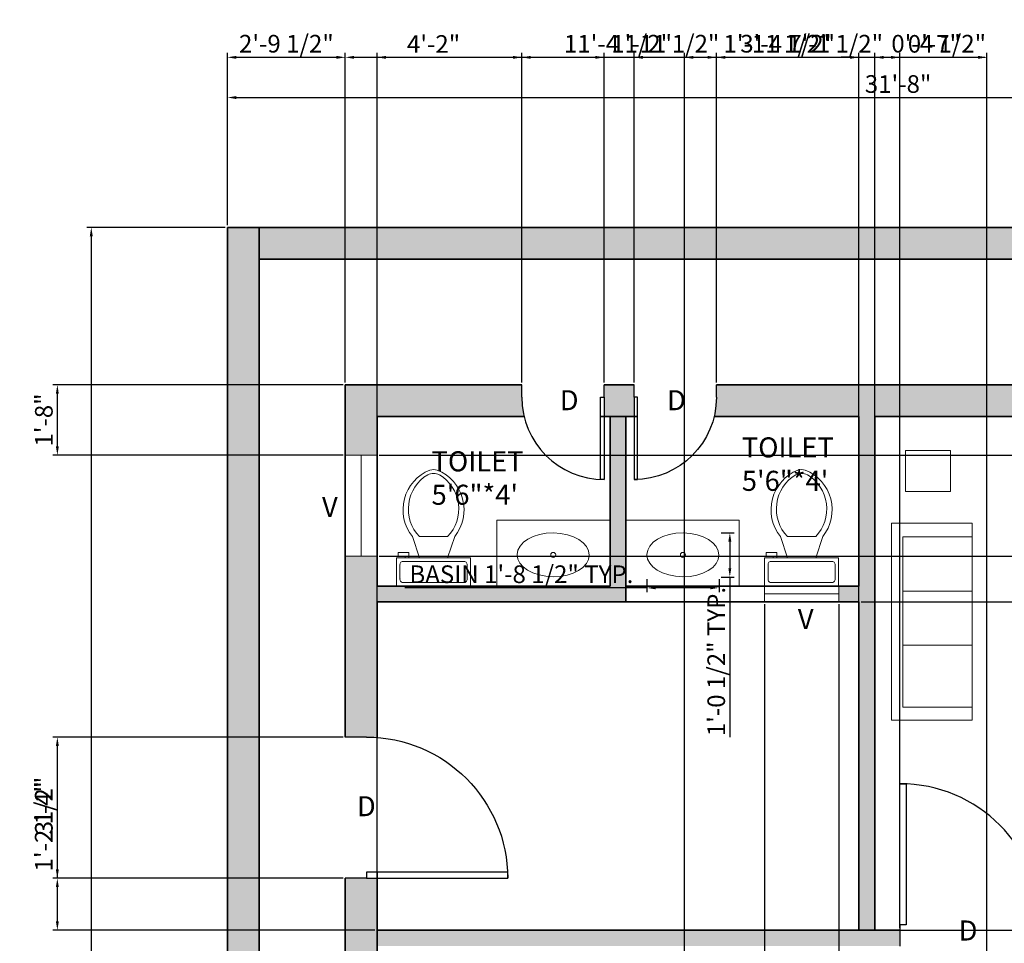
# Model space of a CAD drawing. Units: inches. Extents: x 2130 to 2621, y 981 to 1994.
# Tile 3 of 4: x 2130 to 2409, y 1732 to 1994. Entities that reach past the tile are written whole.
import ezdxf

# ---------------------------------------------------------------- set-up
doc = ezdxf.new("R2010")
doc.units = ezdxf.units.IN
for name, color, linetype, lineweight in [('A-ANNO-DIMS', 2, 'Continuous', 18), ('A-ANNO-TEXT', 10, 'Continuous', 18), ('A-AREA-IDEN', 10, 'Continuous', 18), ('A-FLOR-FIXT', 190, 'Continuous', 18), ('A-WALL-PATT', 140, 'Continuous', 13), ('C-PROP', 7, 'Continuous', 35), ('C-PROP-PATT', 140, 'Continuous', 13), ('DOOR', 130, 'Continuous', 25), ('FUR', 190, 'Continuous', 18), ('WALL', 140, 'Continuous', 35), ('WIND', 210, 'Continuous', 18)]:
    doc.layers.add(name, color=color, linetype=linetype, lineweight=lineweight)
doc.styles.get("Standard").update_dxf_attribs({"font": 'arial.ttf'})
doc.dimstyles.new('ISO-25', dxfattribs={"dimtxt": 5, "dimasz": 2.5, "dimexe": 1.25, "dimexo": 0.625, "dimtad": 1, "dimdec": 0, "dimlunit": 4, "dimtxsty": 'Standard', "dimcen": 2.5, "dimadec": 0, "dimazin": 0, "dimtfac": 1, "dimtdec": 0, "dimtmove": 0, "dimatfit": 3, "dimfxl": 1, "dimarcsym": 0})

# ---------------------------------------------------------------- blocks, each defined once
blk = doc.blocks.new('*U2')
for p, q in [((0, 0), (0, -6)), ((40, 0), (40, -6))]:
    blk.add_line(p, q)
blk.add_lwpolyline([(0, 0), (0, 40), (1.75, 40), (1.75, 0)], close=True)
blk.add_arc((0, 0), 40, 0, 90)
blk = doc.blocks.new('*D9')
at = {"layer": 'A-ANNO-DIMS', "color": 0, "lineweight": -2, "transparency": 16777216}
for p, q in [((2188.76, 1935.64), (2188.76, 1973.06)), ((2568.76, 1935.64), (2568.76, 1973.06)), ((2191.26, 1971.81), (2566.26, 1971.81))]:
    blk.add_line(p, q, dxfattribs=at)
at = {"layer": 'A-ANNO-DIMS', "color": 0, "transparency": 16777216}
for points in [[(2191.26, 1972.23), (2191.26, 1971.39), (2188.76, 1971.81)], [(2566.26, 1972.23), (2566.26, 1971.39), (2568.76, 1971.81)]]:
    blk.add_solid(points, dxfattribs=at)
at = {"layer": 'Defpoints', "color": 0, "transparency": 16777216}
for p in [(2568.76, 1971.81), (2188.76, 1935.02), (2568.76, 1935.02)]:
    blk.add_point(p, dxfattribs=at)
at = {"layer": 'A-ANNO-DIMS', "color": 0, "transparency": 16777216, "insert": (2378.76, 1974.99), "char_height": 5, "attachment_point": 5}
blk.add_mtext('31\'-8"', dxfattribs=at)
blk = doc.blocks.new('*D10')
at = {"layer": 'A-ANNO-DIMS', "color": 0, "lineweight": -2, "transparency": 16777216}
for p, q in [((2188.13, 1935.02), (2148.94, 1935.02)), ((2150.19, 1932.52), (2150.19, 1079.91)), ((2188.13, 1077.41), (2148.94, 1077.41))]:
    blk.add_line(p, q, dxfattribs=at)
at = {"layer": 'A-ANNO-DIMS', "color": 0, "transparency": 16777216}
for points in [[(2149.77, 1932.52), (2150.61, 1932.52), (2150.19, 1935.02)], [(2149.77, 1079.91), (2150.61, 1079.91), (2150.19, 1077.41)]]:
    blk.add_solid(points, dxfattribs=at)
at = {"layer": 'Defpoints', "color": 0, "transparency": 16777216}
for p in [(2188.76, 1935.02), (2150.19, 1077.41), (2188.76, 1077.41)]:
    blk.add_point(p, dxfattribs=at)
at = {"layer": 'A-ANNO-DIMS', "color": 0, "transparency": 16777216, "insert": (2147.01, 1506.21), "char_height": 5, "attachment_point": 5, "rotation": 90}
blk.add_mtext('71\'-6"', dxfattribs=at)
blk = doc.blocks.new('*U4')
for p, q in [((9.5, -6), (9.5, -2)), ((-8, -8.5), (-8, -8)), ((-7, -8), (-7, -9.5)), ((-4, -8), (-6, -14)), ((4, -8), (6, -14)), ((-10, -8.5), (-8, -8.5)), ((-10, -9.5), (-10, -8.5)), ((-7, -9.5), (-10, -9.5)), ((4, -14), (-4, -14))]:
    blk.add_line(p, q)
blk.add_lwpolyline([(10.5, -8), (10.5, 0), (-10.5, 0), (-10.5, -8)], close=True)
for points in [[(-9.5, -2), (-9.5, -6)], [(8.5, -1), (-8.5, -1)], [(-8.5, -7), (8.5, -7)]]:
    blk.add_lwpolyline(points)
for centre, radius, start, end in [((-8.62, -1.88), 0.884, 81.8699, 188.1301), ((8.62, -1.88), 0.884, 351.8699, 98.1301), ((-8.62, -6.12), 0.884, 171.8699, 278.1301), ((8.62, -6.12), 0.884, 261.8699, 8.1301), ((3.52, -21.58), 12.17, 141.4691, 247.9714), ((4.2, -21.82), 11.33, 136.3677, 238.9468), ((-3.52, -21.58), 12.17, 292.0284, 38.5307), ((-4.2, -21.82), 11.33, 301.053, 43.6321), ((0, -27.88), 4, 245.7318, 294.2682), ((0, -29), 4, 254.8605, 285.1395)]:
    blk.add_arc(centre, radius, start, end)
blk = doc.blocks.new('SOFA-THREE-SEAT')
for p, q in [((0, 0), (0, 55.76)), ((0, 55.76), (22.87, 55.76)), ((22.87, 55.76), (22.87, 51.91)), ((3.25, 36.47), (22.87, 36.47)), ((3.25, 21.24), (22.87, 21.24)), ((22.87, 3.65), (22.87, 0)), ((1.57, 0), (0, 0)), ((22.87, 0), (1.57, 0))]:
    blk.add_line(p, q)
blk.add_lwpolyline([(3.25, 3.65), (22.87, 3.65), (22.87, 51.91), (3.25, 51.91)], close=True)
blk = doc.blocks.new('BASIN-OVAL')
blk.add_circle((10.2, 6.23), 0.708)
blk.add_ellipse((10.2, 6.23), major_axis=(10.2, -0.08), ratio=0.610803)
blk = doc.blocks.new('*D19')
at = {"layer": 'A-ANNO-DIMS', "color": 0, "lineweight": -2, "transparency": 16777216}
for p, q in [((2307.57, 1832.9), (2239.01, 1832.9)), ((2307.57, 1835.34), (2307.57, 1831.65)), ((2325.53, 1832.9), (2310.07, 1832.9)), ((2328.03, 1835.34), (2328.03, 1831.65))]:
    blk.add_line(p, q, dxfattribs=at)
at = {"layer": 'A-ANNO-DIMS', "color": 0, "transparency": 16777216}
for points in [[(2310.07, 1833.32), (2310.07, 1832.48), (2307.57, 1832.9)], [(2325.53, 1833.32), (2325.53, 1832.48), (2328.03, 1832.9)]]:
    blk.add_solid(points, dxfattribs=at)
at = {"layer": 'Defpoints', "color": 0, "transparency": 16777216}
for p in [(2307.57, 1835.97), (2328.03, 1835.97), (2307.57, 1832.9)]:
    blk.add_point(p, dxfattribs=at)
at = {"layer": 'A-ANNO-DIMS', "color": 0, "transparency": 16777216, "insert": (2272.04, 1836.11), "char_height": 5, "attachment_point": 5}
blk.add_mtext('BASIN 1\'-8 1/2" TYP.', dxfattribs=at)
blk = doc.blocks.new('*D20')
at = {"layer": 'A-ANNO-DIMS', "color": 0, "lineweight": -2, "transparency": 16777216}
for p, q in [((2328.65, 1848.52), (2332.35, 1848.52)), ((2331.1, 1846.02), (2331.1, 1838.47)), ((2328.65, 1835.97), (2332.35, 1835.97)), ((2331.1, 1835.97), (2331.1, 1790.56))]:
    blk.add_line(p, q, dxfattribs=at)
at = {"layer": 'A-ANNO-DIMS', "color": 0, "transparency": 16777216}
for points in [[(2330.68, 1846.02), (2331.51, 1846.02), (2331.1, 1848.52)], [(2330.68, 1838.47), (2331.51, 1838.47), (2331.1, 1835.97)]]:
    blk.add_solid(points, dxfattribs=at)
at = {"layer": 'Defpoints', "color": 0, "transparency": 16777216}
for p in [(2328.03, 1848.52), (2328.03, 1835.97), (2331.1, 1835.97)]:
    blk.add_point(p, dxfattribs=at)
at = {"layer": 'A-ANNO-DIMS', "color": 0, "transparency": 16777216, "insert": (2327.89, 1812.02), "char_height": 5, "attachment_point": 5, "rotation": 90}
blk.add_mtext('1\'-0 1/2" TYP.', dxfattribs=at)
blk = doc.blocks.new('*D25')
at = {"layer": 'A-ANNO-DIMS', "color": 0, "lineweight": -2, "transparency": 16777216}
for p, q in [((2188.76, 1935.64), (2188.76, 1984.45)), ((2222.16, 1891.04), (2222.16, 1984.45)), ((2191.26, 1983.2), (2219.66, 1983.2))]:
    blk.add_line(p, q, dxfattribs=at)
at = {"layer": 'A-ANNO-DIMS', "color": 0, "transparency": 16777216}
for points in [[(2191.26, 1983.61), (2191.26, 1982.78), (2188.76, 1983.2)], [(2219.66, 1983.61), (2219.66, 1982.78), (2222.16, 1983.2)]]:
    blk.add_solid(points, dxfattribs=at)
at = {"layer": 'Defpoints', "color": 0, "transparency": 16777216}
for p in [(2222.16, 1983.2), (2188.76, 1935.02), (2222.16, 1890.41)]:
    blk.add_point(p, dxfattribs=at)
at = {"layer": 'A-ANNO-DIMS', "color": 0, "transparency": 16777216, "insert": (2205.46, 1986.41), "char_height": 5, "attachment_point": 5}
blk.add_mtext('2\'-9 1/2"', dxfattribs=at)
blk = doc.blocks.new('*D28')
at = {"layer": 'A-ANNO-DIMS', "color": 0, "lineweight": -2, "transparency": 16777216}
for p, q in [((2231.16, 1736.54), (2231.16, 1984.45)), ((2367.66, 1736.54), (2367.66, 1984.45)), ((2233.66, 1983.2), (2365.16, 1983.2))]:
    blk.add_line(p, q, dxfattribs=at)
at = {"layer": 'A-ANNO-DIMS', "color": 0, "transparency": 16777216}
for points in [[(2233.66, 1983.61), (2233.66, 1982.78), (2231.16, 1983.2)], [(2365.16, 1983.61), (2365.16, 1982.78), (2367.66, 1983.2)]]:
    blk.add_solid(points, dxfattribs=at)
at = {"layer": 'Defpoints', "color": 0, "transparency": 16777216}
for p in [(2367.66, 1983.2), (2231.16, 1735.91), (2367.66, 1735.91)]:
    blk.add_point(p, dxfattribs=at)
at = {"layer": 'A-ANNO-DIMS', "color": 0, "transparency": 16777216, "insert": (2299.41, 1986.41), "char_height": 5, "attachment_point": 5}
blk.add_mtext('11\'-4 1/2"', dxfattribs=at)
blk = doc.blocks.new('*D29')
at = {"layer": 'A-ANNO-DIMS', "color": 0, "lineweight": -2, "transparency": 16777216}
for p, q in [((2368.29, 1828.91), (2618.19, 1828.91)), ((2616.94, 1738.41), (2616.94, 1826.41)), ((2368.29, 1735.91), (2618.19, 1735.91))]:
    blk.add_line(p, q, dxfattribs=at)
at = {"layer": 'A-ANNO-DIMS', "color": 0, "transparency": 16777216}
for points in [[(2616.52, 1826.41), (2617.35, 1826.41), (2616.94, 1828.91)], [(2616.52, 1738.41), (2617.35, 1738.41), (2616.94, 1735.91)]]:
    blk.add_solid(points, dxfattribs=at)
at = {"layer": 'Defpoints', "color": 0, "transparency": 16777216}
for p in [(2367.66, 1828.91), (2616.94, 1828.91), (2367.66, 1735.91)]:
    blk.add_point(p, dxfattribs=at)
at = {"layer": 'A-ANNO-DIMS', "color": 0, "transparency": 16777216, "insert": (2613.76, 1782.41), "char_height": 5, "attachment_point": 5, "rotation": 90}
blk.add_mtext('7\'-9"', dxfattribs=at)
blk = doc.blocks.new('*D32')
at = {"layer": 'A-ANNO-DIMS', "color": 0, "lineweight": -2, "transparency": 16777216}
for p, q in [((2318.23, 1585.04), (2318.23, 1984.45)), ((2403.94, 1585.04), (2403.94, 1984.45)), ((2320.73, 1983.2), (2401.44, 1983.2))]:
    blk.add_line(p, q, dxfattribs=at)
at = {"layer": 'A-ANNO-DIMS', "color": 0, "transparency": 16777216}
for points in [[(2320.73, 1983.61), (2320.73, 1982.78), (2318.23, 1983.2)], [(2401.44, 1983.61), (2401.44, 1982.78), (2403.94, 1983.2)]]:
    blk.add_solid(points, dxfattribs=at)
at = {"layer": 'Defpoints', "color": 0, "transparency": 16777216}
for p in [(2403.94, 1983.2), (2318.23, 1584.41), (2403.94, 1584.41)]:
    blk.add_point(p, dxfattribs=at)
at = {"layer": 'A-ANNO-DIMS', "color": 0, "transparency": 16777216, "insert": (2361.08, 1986.41), "char_height": 5, "attachment_point": 5}
blk.add_mtext('7\'-1 1/2"', dxfattribs=at)
blk = doc.blocks.new('*D34')
at = {"layer": 'A-ANNO-DIMS', "color": 0, "lineweight": -2, "transparency": 16777216}
for p, q in [((2272.17, 1891.04), (2272.17, 1984.45)), ((2295.51, 1891.04), (2295.51, 1984.45)), ((2274.67, 1983.2), (2293.01, 1983.2)), ((2295.51, 1983.2), (2327.62, 1983.2))]:
    blk.add_line(p, q, dxfattribs=at)
at = {"layer": 'A-ANNO-DIMS', "color": 0, "transparency": 16777216}
for points in [[(2274.67, 1983.61), (2274.67, 1982.78), (2272.17, 1983.2)], [(2293.01, 1983.61), (2293.01, 1982.78), (2295.51, 1983.2)]]:
    blk.add_solid(points, dxfattribs=at)
at = {"layer": 'Defpoints', "color": 0, "transparency": 16777216}
for p in [(2295.51, 1983.2), (2272.17, 1890.41), (2295.51, 1890.41)]:
    blk.add_point(p, dxfattribs=at)
at = {"layer": 'A-ANNO-DIMS', "color": 0, "transparency": 16777216, "insert": (2312.81, 1986.41), "char_height": 5, "attachment_point": 5}
blk.add_mtext('1\'-11 1/2"', dxfattribs=at)
blk = doc.blocks.new('*D35')
at = {"layer": 'A-ANNO-DIMS', "color": 0, "lineweight": -2, "transparency": 16777216}
for p, q in [((2221.54, 1790.61), (2139.33, 1790.61)), ((2140.58, 1753.11), (2140.58, 1788.11)), ((2221.54, 1750.61), (2139.33, 1750.61))]:
    blk.add_line(p, q, dxfattribs=at)
at = {"layer": 'A-ANNO-DIMS', "color": 0, "transparency": 16777216}
for points in [[(2140.16, 1788.11), (2140.99, 1788.11), (2140.58, 1790.61)], [(2140.16, 1753.11), (2140.99, 1753.11), (2140.58, 1750.61)]]:
    blk.add_solid(points, dxfattribs=at)
at = {"layer": 'Defpoints', "color": 0, "transparency": 16777216}
for p in [(2140.58, 1790.61), (2222.16, 1790.61), (2222.16, 1750.61)]:
    blk.add_point(p, dxfattribs=at)
at = {"layer": 'A-ANNO-DIMS', "color": 0, "transparency": 16777216, "insert": (2137.4, 1770.61), "char_height": 5, "attachment_point": 5, "rotation": 90}
blk.add_mtext('3\'-4"', dxfattribs=at)
blk = doc.blocks.new('*D41')
at = {"layer": 'A-ANNO-DIMS', "color": 0, "lineweight": -2, "transparency": 16777216}
for p, q in [((2222.16, 1891.04), (2222.16, 1984.45)), ((2272.17, 1891.04), (2272.17, 1984.45)), ((2224.66, 1983.2), (2269.67, 1983.2))]:
    blk.add_line(p, q, dxfattribs=at)
at = {"layer": 'A-ANNO-DIMS', "color": 0, "transparency": 16777216}
for points in [[(2224.66, 1983.61), (2224.66, 1982.78), (2222.16, 1983.2)], [(2269.67, 1983.61), (2269.67, 1982.78), (2272.17, 1983.2)]]:
    blk.add_solid(points, dxfattribs=at)
at = {"layer": 'Defpoints', "color": 0, "transparency": 16777216}
for p in [(2272.17, 1983.2), (2222.16, 1890.41), (2272.17, 1890.41)]:
    blk.add_point(p, dxfattribs=at)
at = {"layer": 'A-ANNO-DIMS', "color": 0, "transparency": 16777216, "insert": (2247.16, 1986.33), "char_height": 5, "attachment_point": 5}
blk.add_mtext('4\'-2"', dxfattribs=at)
blk = doc.blocks.new('*D43')
at = {"layer": 'A-ANNO-DIMS', "color": 0, "lineweight": -2, "transparency": 16777216}
for p, q in [((2231.79, 1870.49), (2618.19, 1870.49)), ((2616.94, 1844.36), (2616.94, 1867.99)), ((2231.79, 1841.86), (2618.19, 1841.86))]:
    blk.add_line(p, q, dxfattribs=at)
at = {"layer": 'A-ANNO-DIMS', "color": 0, "transparency": 16777216}
for points in [[(2616.52, 1867.99), (2617.35, 1867.99), (2616.94, 1870.49)], [(2616.52, 1844.36), (2617.35, 1844.36), (2616.94, 1841.86)]]:
    blk.add_solid(points, dxfattribs=at)
at = {"layer": 'Defpoints', "color": 0, "transparency": 16777216}
for p in [(2231.16, 1870.49), (2616.94, 1870.49), (2231.16, 1841.86)]:
    blk.add_point(p, dxfattribs=at)
at = {"layer": 'A-ANNO-DIMS', "color": 0, "transparency": 16777216, "insert": (2613.73, 1856.18), "char_height": 5, "attachment_point": 5, "rotation": 90}
blk.add_mtext('2\'-4 1/2"', dxfattribs=at)
blk = doc.blocks.new('*D45')
at = {"layer": 'A-ANNO-DIMS', "color": 0, "lineweight": -2, "transparency": 16777216}
for p, q in [((2340.91, 1828.29), (2340.91, 984.42)), ((2361.98, 1828.29), (2361.98, 984.42)), ((2343.41, 985.67), (2359.48, 985.67))]:
    blk.add_line(p, q, dxfattribs=at)
at = {"layer": 'A-ANNO-DIMS', "color": 0, "transparency": 16777216}
for points in [[(2343.41, 986.08), (2343.41, 985.25), (2340.91, 985.67)], [(2359.48, 986.08), (2359.48, 985.25), (2361.98, 985.67)]]:
    blk.add_solid(points, dxfattribs=at)
at = {"layer": 'Defpoints', "color": 0, "transparency": 16777216}
for p in [(2340.91, 1828.91), (2361.98, 1828.91), (2361.98, 985.67)]:
    blk.add_point(p, dxfattribs=at)
at = {"layer": 'A-ANNO-DIMS', "color": 0, "transparency": 16777216, "insert": (2351.44, 988.84), "char_height": 5, "attachment_point": 5}
blk.add_mtext('1\'-9"', dxfattribs=at)
blk = doc.blocks.new('*D46')
at = {"layer": 'A-ANNO-DIMS', "color": 0, "lineweight": -2, "transparency": 16777216}
for p, q in [((2140.58, 1750.61), (2140.58, 1778.83)), ((2221.54, 1750.61), (2139.33, 1750.61)), ((2140.58, 1738.41), (2140.58, 1748.11)), ((2230.54, 1735.91), (2139.33, 1735.91))]:
    blk.add_line(p, q, dxfattribs=at)
at = {"layer": 'A-ANNO-DIMS', "color": 0, "transparency": 16777216}
for points in [[(2140.16, 1748.11), (2140.99, 1748.11), (2140.58, 1750.61)], [(2140.16, 1738.41), (2140.99, 1738.41), (2140.58, 1735.91)]]:
    blk.add_solid(points, dxfattribs=at)
at = {"layer": 'Defpoints', "color": 0, "transparency": 16777216}
for p in [(2140.58, 1750.61), (2222.16, 1750.61), (2231.16, 1735.91)]:
    blk.add_point(p, dxfattribs=at)
at = {"layer": 'A-ANNO-DIMS', "color": 0, "transparency": 16777216, "insert": (2137.37, 1765.97), "char_height": 5, "attachment_point": 5, "rotation": 90}
blk.add_mtext('1\'-2 1/2"', dxfattribs=at)
blk = doc.blocks.new('*D48')
at = {"layer": 'A-ANNO-DIMS', "color": 0, "lineweight": -2, "transparency": 16777216}
for p, q in [((2327.29, 1891.04), (2327.29, 1984.45)), ((2367.66, 1882.04), (2367.66, 1984.45)), ((2329.79, 1983.2), (2365.16, 1983.2))]:
    blk.add_line(p, q, dxfattribs=at)
at = {"layer": 'A-ANNO-DIMS', "color": 0, "transparency": 16777216}
for points in [[(2329.79, 1983.61), (2329.79, 1982.78), (2327.29, 1983.2)], [(2365.16, 1983.61), (2365.16, 1982.78), (2367.66, 1983.2)]]:
    blk.add_solid(points, dxfattribs=at)
at = {"layer": 'Defpoints', "color": 0, "transparency": 16777216}
for p in [(2367.66, 1983.2), (2327.29, 1890.41), (2367.66, 1881.41)]:
    blk.add_point(p, dxfattribs=at)
at = {"layer": 'A-ANNO-DIMS', "color": 0, "transparency": 16777216, "insert": (2347.47, 1986.41), "char_height": 5, "attachment_point": 5}
blk.add_mtext('3\'-4 1/2"', dxfattribs=at)
blk = doc.blocks.new('*D50')
at = {"layer": 'A-ANNO-DIMS', "color": 0, "lineweight": -2, "transparency": 16777216}
for p, q in [((2367.66, 1736.54), (2367.66, 1984.45)), ((2372.16, 1736.54), (2372.16, 1984.45)), ((2365.16, 1983.2), (2362.66, 1983.2)), ((2367.66, 1983.2), (2372.16, 1983.2)), ((2374.66, 1983.2), (2403.35, 1983.2))]:
    blk.add_line(p, q, dxfattribs=at)
at = {"layer": 'A-ANNO-DIMS', "color": 0, "transparency": 16777216}
for points in [[(2365.16, 1983.61), (2365.16, 1982.78), (2367.66, 1983.2)], [(2374.66, 1983.61), (2374.66, 1982.78), (2372.16, 1983.2)]]:
    blk.add_solid(points, dxfattribs=at)
at = {"layer": 'Defpoints', "color": 0, "transparency": 16777216}
for p in [(2372.16, 1983.2), (2367.66, 1735.91), (2372.16, 1735.91)]:
    blk.add_point(p, dxfattribs=at)
at = {"layer": 'A-ANNO-DIMS', "color": 0, "transparency": 16777216, "insert": (2390.26, 1986.41), "char_height": 5, "attachment_point": 5}
blk.add_mtext('0\'-4 1/2"', dxfattribs=at)
blk = doc.blocks.new('*D51')
at = {"layer": 'A-ANNO-DIMS', "color": 0, "lineweight": -2, "transparency": 16777216}
for p, q in [((2303.95, 1891.04), (2303.95, 1984.45)), ((2327.29, 1891.04), (2327.29, 1984.45)), ((2306.45, 1983.2), (2324.79, 1983.2)), ((2327.29, 1983.2), (2359.4, 1983.2))]:
    blk.add_line(p, q, dxfattribs=at)
at = {"layer": 'A-ANNO-DIMS', "color": 0, "transparency": 16777216}
for points in [[(2306.45, 1983.61), (2306.45, 1982.78), (2303.95, 1983.2)], [(2324.79, 1983.61), (2324.79, 1982.78), (2327.29, 1983.2)]]:
    blk.add_solid(points, dxfattribs=at)
at = {"layer": 'Defpoints', "color": 0, "transparency": 16777216}
for p in [(2327.29, 1983.2), (2303.95, 1890.41), (2327.29, 1890.41)]:
    blk.add_point(p, dxfattribs=at)
at = {"layer": 'A-ANNO-DIMS', "color": 0, "transparency": 16777216, "insert": (2344.59, 1986.41), "char_height": 5, "attachment_point": 5}
blk.add_mtext('1\'-11 1/2"', dxfattribs=at)
blk = doc.blocks.new('*D52')
at = {"layer": 'A-ANNO-DIMS', "color": 0, "lineweight": -2, "transparency": 16777216}
for p, q in [((2372.16, 1736.54), (2372.16, 1984.45)), ((2379.27, 1736.54), (2379.27, 1984.45)), ((2374.66, 1983.2), (2376.77, 1983.2)), ((2379.27, 1983.2), (2396.31, 1983.2))]:
    blk.add_line(p, q, dxfattribs=at)
at = {"layer": 'A-ANNO-DIMS', "color": 0, "transparency": 16777216}
for points in [[(2374.66, 1983.61), (2374.66, 1982.78), (2372.16, 1983.2)], [(2376.77, 1983.61), (2376.77, 1982.78), (2379.27, 1983.2)]]:
    blk.add_solid(points, dxfattribs=at)
at = {"layer": 'Defpoints', "color": 0, "transparency": 16777216}
for p in [(2379.27, 1983.2), (2372.16, 1735.91), (2379.27, 1735.91)]:
    blk.add_point(p, dxfattribs=at)
at = {"layer": 'A-ANNO-DIMS', "color": 0, "transparency": 16777216, "insert": (2389.04, 1986.37), "char_height": 5, "attachment_point": 5}
blk.add_mtext('0\'-7"', dxfattribs=at)
blk = doc.blocks.new('*D55')
at = {"layer": 'A-ANNO-DIMS', "color": 0, "lineweight": -2, "transparency": 16777216}
for p, q in [((2221.54, 1890.41), (2139.33, 1890.41)), ((2140.58, 1872.99), (2140.58, 1887.91)), ((2221.54, 1870.49), (2139.33, 1870.49))]:
    blk.add_line(p, q, dxfattribs=at)
at = {"layer": 'A-ANNO-DIMS', "color": 0, "transparency": 16777216}
for points in [[(2140.16, 1887.91), (2140.99, 1887.91), (2140.58, 1890.41)], [(2140.16, 1872.99), (2140.99, 1872.99), (2140.58, 1870.49)]]:
    blk.add_solid(points, dxfattribs=at)
at = {"layer": 'Defpoints', "color": 0, "transparency": 16777216}
for p in [(2140.58, 1890.41), (2222.16, 1890.41), (2222.16, 1870.49)]:
    blk.add_point(p, dxfattribs=at)
at = {"layer": 'A-ANNO-DIMS', "color": 0, "transparency": 16777216, "insert": (2137.4, 1880.45), "char_height": 5, "attachment_point": 5, "rotation": 90}
blk.add_mtext('1\'-8"', dxfattribs=at)

msp = doc.modelspace()

# ---------------------------------------------------------------- hatches: boundary and pattern name
at = {"layer": 'A-WALL-PATT'}
h = msp.add_hatch(color=256, dxfattribs=at)
h.dxf.hatch_style = 1
h.paths.add_polyline_path([(2272.17, 1886.91), (2272.17, 1890.41), (2222.16, 1890.41), (2222.16, 1870.49), (2231.16, 1870.49), (2231.16, 1881.41), (2272.82, 1881.41, -0.059514)])
h.paths.add_polyline_path([(2231.16, 1828.91), (2301.66, 1828.91), (2301.66, 1881.41), (2297.16, 1881.41), (2297.16, 1833.41), (2265.07, 1833.41), (2231.16, 1833.41), (2231.16, 1841.86), (2222.16, 1841.86), (2222.16, 1828.91), (2222.16, 1790.61), (2228.16, 1790.61, -0.01877), (2231.16, 1790.5)])
h.paths.add_polyline_path([(2303.95, 1886.91), (2303.95, 1890.41), (2301.66, 1890.41), (2295.51, 1890.41), (2295.51, 1886.91), (2295.51, 1881.41), (2297.16, 1881.41), (2301.66, 1881.41), (2303.95, 1881.41)])
h.paths.add_polyline_path([(2525.16, 1890.41), (2372.16, 1890.41), (2327.29, 1890.41), (2327.29, 1886.91, -0.059514), (2326.63, 1881.41), (2367.66, 1881.41), (2367.66, 1833.41), (2361.98, 1833.41), (2361.98, 1828.91), (2367.66, 1828.91), (2367.66, 1735.91), (2372.16, 1735.91), (2372.16, 1828.91), (2372.16, 1881.41), (2516.16, 1881.41), (2516.16, 1859.91), (2516.16, 1809.41), (2525.16, 1809.41)])
h.paths.add_polyline_path([(2475.37, 1735.91), (2419.27, 1735.91), (2419.27, 1731.41), (2475.37, 1731.41), (2475.37, 1731.77)])
h.paths.add_polyline_path([(2525.16, 1751.59), (2516.16, 1751.59), (2516.16, 1737.41), (2516.16, 1735.91), (2503, 1735.91), (2503, 1731.77, -0.030428), (2502.8, 1728.41), (2516.16, 1728.41), (2516.16, 1714.24), (2525.16, 1714.24), (2525.16, 1728.41)])
h.paths.add_polyline_path([(2379.27, 1735.91), (2231.16, 1735.91), (2231.16, 1731.41), (2379.27, 1731.41)])
h.paths.add_polyline_path([(2231.16, 1728.41), (2231.16, 1735.91), (2231.16, 1750.61), (2228.16, 1750.61), (2222.16, 1750.61), (2222.16, 1728.41), (2222.16, 1674.58), (2231.16, 1674.58)])
h.paths.add_polyline_path([(2516.16, 1584.41), (2462.16, 1584.41), (2403.94, 1584.41), (2403.94, 1575.41), (2404.07, 1575.41), (2453.16, 1575.41), (2516.16, 1575.41)], flags=17)
h.paths.add_polyline_path([(2516.16, 1584.41), (2462.16, 1584.41), (2403.94, 1584.41), (2403.94, 1575.41), (2453.16, 1575.41), (2516.16, 1575.41)], flags=17)
h.paths.add_polyline_path([(2318.23, 1584.41), (2231.16, 1584.41), (2231.16, 1575.41), (2318.23, 1575.41)])
h = msp.add_hatch(color=256, dxfattribs=at)
h.dxf.hatch_style = 1
h.paths.add_polyline_path([(2231.16, 1595.8), (2222.16, 1595.8), (2222.16, 1571.6), (2225.81, 1571.6), (2231.16, 1571.6)])
h.paths.add_polyline_path([(2313.28, 1362.41), (2237.26, 1362.41), (2231.16, 1362.41), (2231.16, 1404.41), (2231.16, 1474.85), (2231.16, 1547.86, -0.05547), (2225.81, 1547.27), (2222.16, 1547.27), (2222.16, 1425.41), (2222.16, 1353.41), (2313.28, 1353.41)])
h.paths.add_polyline_path([(2393.01, 1195.09), (2434.46, 1195.09), (2434.46, 1216.28), (2393.01, 1216.28)], flags=9)
h.paths.add_polyline_path([(2245.08, 1335), (2303.47, 1335), (2303.47, 1346.7), (2245.08, 1346.7)], flags=9)
h.paths.add_polyline_path([(2458.81, 1338.38), (2517.21, 1338.38), (2517.21, 1350.09), (2458.81, 1350.09)], flags=9)
h.paths.add_polyline_path([(2232.7, 1530.42), (2263.31, 1530.42), (2263.31, 1551.62), (2232.7, 1551.62)], flags=9)
h.paths.add_polyline_path([(2332.94, 1458.61), (2399.05, 1458.61), (2399.05, 1489.37), (2332.94, 1489.37)], flags=9)
h.paths.add_polyline_path([(2475.66, 1607.66), (2507.9, 1607.66), (2507.9, 1628.85), (2475.66, 1628.85)], flags=9)
h.paths.add_polyline_path([(2486.7, 1688.97), (2517.32, 1688.97), (2517.32, 1710.17), (2486.7, 1710.17)], flags=9)
h.paths.add_polyline_path([(2333.88, 1649.81), (2375.07, 1649.81), (2375.07, 1671), (2333.88, 1671)], flags=9)
h.paths.add_polyline_path([(2441.42, 1774.34), (2500.24, 1774.34), (2500.24, 1795.53), (2441.42, 1795.53)], flags=9)
h.paths.add_polyline_path([(2332.74, 1857.16), (2363.5, 1857.16), (2363.5, 1878.35), (2332.74, 1878.35)], flags=9)
h.paths.add_polyline_path([(2244.84, 1853.21), (2275.6, 1853.21), (2275.6, 1874.4), (2244.84, 1874.4)], flags=9)
at = {"layer": 'C-PROP-PATT'}
h = msp.add_hatch(color=256, dxfattribs=at)
h.dxf.hatch_style = 1
h.paths.add_polyline_path([(2559.76, 1935.02), (2197.76, 1935.02), (2197.76, 1926.02), (2559.76, 1926.02)])
h.paths.add_polyline_path([(2197.76, 1935.02), (2188.76, 1935.02), (2188.76, 1077.41), (2197.76, 1077.41)])
h.paths.add_polyline_path([(2568.76, 1926.02), (2559.76, 1926.02), (2559.76, 1077.41), (2568.76, 1077.41)])
h.paths.add_polyline_path([(2568.76, 1935.02), (2559.76, 1935.02), (2559.76, 1926.02), (2568.76, 1926.02)])

# ---------------------------------------------------------------- linework, layer by layer
at = {"layer": 'A-FLOR-FIXT'}
for points in [[(2297.16, 1833.41), (2265.07, 1833.41), (2265.07, 1852.04), (2297.16, 1852.04)], [(2333.75, 1833.41), (2301.66, 1833.41), (2301.66, 1852.04), (2333.75, 1852.04)]]:
    msp.add_lwpolyline(points, close=True, dxfattribs=at)
at = {"layer": 'C-PROP'}
for p, q in [((2188.76, 1935.02), (2188.76, 1077.41)), ((2188.76, 1935.02), (2568.76, 1935.02)), ((2197.76, 1926.02), (2559.76, 1926.02)), ((2197.76, 1926.02), (2197.76, 1086.41))]:
    msp.add_line(p, q, dxfattribs=at)
for points in [[(2188.76, 1935.02), (2197.76, 1935.02), (2197.76, 1077.41), (2188.76, 1077.41)], [(2197.76, 1926.02), (2568.76, 1926.02), (2568.76, 1935.02), (2197.76, 1935.02)]]:
    msp.add_lwpolyline(points, close=True, dxfattribs=at)
at = {"layer": 'FUR'}
msp.add_lwpolyline([(2380.9, 1871.79), (2393.64, 1871.79), (2393.64, 1860.19), (2380.9, 1860.19)], close=True, dxfattribs=at)
at = {"layer": 'WALL'}
for p, q in [((2222.16, 1890.41), (2272.17, 1890.41)), ((2222.16, 1890.41), (2222.16, 1828.91)), ((2295.51, 1890.41), (2301.66, 1890.41)), ((2301.66, 1890.41), (2303.95, 1890.41)), ((2327.29, 1890.41), (2372.16, 1890.41)), ((2372.16, 1890.41), (2525.16, 1890.41)), ((2231.16, 1881.41), (2272.82, 1881.41)), ((2231.16, 1881.41), (2231.16, 1833.41)), ((2294.49, 1881.41), (2297.16, 1881.41)), ((2297.16, 1833.41), (2297.16, 1881.41)), ((2297.16, 1881.41), (2301.66, 1881.41)), ((2301.66, 1828.91), (2301.66, 1881.41)), ((2301.66, 1881.41), (2304.97, 1881.41)), ((2326.63, 1881.41), (2367.66, 1881.41)), ((2367.66, 1881.41), (2367.66, 1833.41)), ((2372.16, 1881.41), (2372.16, 1828.91)), ((2372.16, 1881.41), (2516.16, 1881.41)), ((2231.16, 1833.41), (2297.16, 1833.41)), ((2367.66, 1833.41), (2301.66, 1833.41)), ((2222.16, 1828.91), (2222.16, 1790.61)), ((2231.16, 1828.91), (2301.66, 1828.91)), ((2231.16, 1828.91), (2231.16, 1790.5)), ((2367.66, 1828.91), (2301.66, 1828.91)), ((2367.66, 1828.91), (2367.66, 1735.91)), ((2367.66, 1735.91), (2367.66, 1828.91)), ((2372.16, 1735.91), (2372.16, 1828.91)), ((2231.16, 1752.36), (2231.16, 1735.91)), ((2222.16, 1750.61), (2222.16, 1728.41)), ((2231.16, 1735.91), (2231.16, 1674.58)), ((2367.66, 1735.91), (2231.16, 1735.91)), ((2231.16, 1735.91), (2379.27, 1735.91))]:
    msp.add_line(p, q, dxfattribs=at)
at = {"layer": 'WIND'}
for p, q in [((2226.66, 1841.86), (2226.66, 1870.49)), ((2340.91, 1831.16), (2361.98, 1831.16))]:
    msp.add_line(p, q, dxfattribs=at)
for points in [[(2231.16, 1841.86), (2222.16, 1841.86), (2222.16, 1870.49), (2231.16, 1870.49)], [(2340.91, 1833.41), (2361.98, 1833.41), (2361.98, 1828.91), (2340.91, 1828.91)]]:
    msp.add_lwpolyline(points, close=True, dxfattribs=at)

# ---------------------------------------------------------------- block references
at = {"layer": 'A-FLOR-FIXT', "xscale": -1, "rotation": 180}
for p in [(2247.15, 1833.41), (2351.41, 1833.41)]:
    msp.add_blockref('*U4', p, dxfattribs=at)
at = {"layer": 'A-FLOR-FIXT'}
msp.add_blockref('BASIN-OVAL', (2270.86, 1836.02), dxfattribs=at)
at = {"layer": 'A-FLOR-FIXT', "rotation": 180}
msp.add_blockref('BASIN-OVAL', (2328, 1848.48), dxfattribs=at)
at = {"layer": 'DOOR', "yscale": 0.5835973235753805, "zscale": 0.5835973235753805, "rotation": 180}
for p, xscale in [((2295.51, 1886.91), 0.5835973235753805), ((2303.95, 1886.91), -0.5835973235753805)]:
    msp.add_blockref('*U2', p, dxfattribs=dict(at, xscale=xscale))
at = {"layer": 'DOOR', "xscale": -1, "rotation": 270}
msp.add_blockref('*U2', (2228.16, 1750.61), dxfattribs=at)
at = {"layer": 'DOOR'}
msp.add_blockref('*U2', (2379.27, 1737.41), dxfattribs=at)
at = {"layer": 'FUR'}
msp.add_blockref('SOFA-THREE-SEAT', (2376.88, 1795.46), dxfattribs=at)

# ---------------------------------------------------------------- texts
at = {"layer": 'A-ANNO-TEXT', "char_height": 5.68, "attachment_point": 1}
for s, insert in [('D', (2282.91, 1888.9)), ('D', (2313.29, 1888.9)), ('V', (2215.55, 1858.68)), ('V', (2350.36, 1826.92)), ('D', (2225.44, 1773.88)), ('D', (2395.92, 1738.66))]:
    msp.add_mtext_dynamic_manual_height_columns(s, width=39.9661, gutter_width=28.4, heights=[0], dxfattribs=dict(at, insert=insert))
at = {"layer": 'A-AREA-IDEN', "char_height": 5.68, "attachment_point": 1}
for insert in [(2334.49, 1875.53), (2246.59, 1871.58)]:
    msp.add_mtext_dynamic_manual_height_columns('TOILET\\P5\'6"*4\'', width=39.9661, gutter_width=28.4, heights=[0], dxfattribs=dict(at, insert=insert))

# ---------------------------------------------------------------- dimensions: what is measured, and where the dimension line sits
at = {"layer": 'A-ANNO-DIMS'}
for base, p1, p2, override, picture, middle in [((2222.16, 1983.2), (2188.76, 1935.02), (2222.16, 1890.41), {"dimdec": 1, "dimlfac": 1, "dimrnd": 0, "dimzin": 1, "dimdsep": 46, "dimlunit": 4, "dimfrac": 2}, '*D25', (2205.46, 1986.41)), ((2367.66, 1983.2), (2231.16, 1735.91), (2367.66, 1735.91), {"dimdec": 1, "dimlfac": 1, "dimrnd": 0, "dimzin": 1, "dimdsep": 46, "dimlunit": 4, "dimfrac": 2}, '*D28', (2299.41, 1986.41)), ((2295.51, 1983.2), (2272.17, 1890.41), (2295.51, 1890.41), {"dimdec": 1, "dimlfac": 1, "dimrnd": 0, "dimzin": 1, "dimdsep": 46, "dimlunit": 4, "dimfrac": 2}, '*D34', (2312.81, 1986.41)), ((2327.29, 1983.2), (2303.95, 1890.41), (2327.29, 1890.41), {"dimdec": 1, "dimlfac": 1, "dimrnd": 0, "dimzin": 1, "dimdsep": 46, "dimlunit": 4, "dimfrac": 2}, '*D51', (2344.59, 1986.41)), ((2403.94, 1983.2), (2318.23, 1584.41), (2403.94, 1584.41), {"dimdec": 1, "dimlfac": 1, "dimrnd": 0, "dimzin": 1, "dimdsep": 46, "dimlunit": 4, "dimfrac": 2}, '*D32', (2361.08, 1986.41)), ((2367.66, 1983.2), (2327.29, 1890.41), (2367.66, 1881.41), {"dimdec": 1, "dimlfac": 1, "dimrnd": 0, "dimzin": 1, "dimdsep": 46, "dimlunit": 4, "dimfrac": 2}, '*D48', (2347.47, 1986.41)), ((2372.16, 1983.2), (2367.66, 1735.91), (2372.16, 1735.91), {"dimdec": 1, "dimlfac": 1, "dimrnd": 0, "dimzin": 1, "dimdsep": 46, "dimlunit": 4, "dimfrac": 2}, '*D50', (2390.26, 1986.41)), ((2272.17, 1983.2), (2222.16, 1890.41), (2272.17, 1890.41), {"dimdec": 1, "dimlfac": 1, "dimrnd": 0, "dimzin": 1, "dimdsep": 46, "dimlunit": 4, "dimfrac": 2}, '*D41', (2247.16, 1986.33)), ((2379.27, 1983.2), (2372.16, 1735.91), (2379.27, 1735.91), {"dimdec": 1, "dimlfac": 1, "dimrnd": 0, "dimzin": 1, "dimdsep": 46, "dimlunit": 4, "dimfrac": 2}, '*D52', (2389.04, 1986.37)), ((2568.76, 1971.81), (2188.76, 1935.02), (2568.76, 1935.02), {"dimclrd": 0, "dimclre": 0, "dimclrt": 0}, '*D9', (2378.76, 1974.99)), ((2361.98, 985.67), (2340.91, 1828.91), (2361.98, 1828.91), {"dimdec": 1, "dimlfac": 1, "dimrnd": 0, "dimzin": 1, "dimdsep": 46, "dimlunit": 4, "dimfrac": 2}, '*D45', (2351.44, 988.84))]:
    dim = msp.add_linear_dim(base=base, p1=p1, p2=p2, dimstyle='ISO-25', override=override, dxfattribs=at)
    dim.commit()
    dim.dimension.update_dxf_attribs({"geometry": picture, "text_midpoint": middle})
for base, p1, p2, override, picture, middle in [((2150.19, 1077.41), (2188.76, 1935.02), (2188.76, 1077.41), {"dimclrd": 0, "dimclre": 0, "dimclrt": 0}, '*D10', (2147.01, 1506.21)), ((2140.58, 1890.41), (2222.16, 1870.49), (2222.16, 1890.41), {"dimdec": 1, "dimlfac": 1, "dimrnd": 0, "dimzin": 1, "dimdsep": 46, "dimlunit": 4, "dimfrac": 2}, '*D55', (2137.4, 1880.45)), ((2616.94, 1870.49), (2231.16, 1841.86), (2231.16, 1870.49), {"dimdec": 1, "dimlfac": 1, "dimrnd": 0, "dimzin": 1, "dimdsep": 46, "dimlunit": 4, "dimfrac": 2}, '*D43', (2613.73, 1856.18)), ((2616.94, 1828.91), (2367.66, 1735.91), (2367.66, 1828.91), {"dimdec": 1, "dimlfac": 1, "dimrnd": 0, "dimzin": 1, "dimdsep": 46, "dimlunit": 4, "dimfrac": 2}, '*D29', (2613.76, 1782.41)), ((2140.58, 1790.61), (2222.16, 1750.61), (2222.16, 1790.61), {"dimdec": 1, "dimlfac": 1, "dimrnd": 0, "dimzin": 1, "dimdsep": 46, "dimlunit": 4, "dimfrac": 2}, '*D35', (2137.4, 1770.61)), ((2140.58, 1750.61), (2231.16, 1735.91), (2222.16, 1750.61), {"dimdec": 1, "dimlfac": 1, "dimrnd": 0, "dimzin": 1, "dimdsep": 46, "dimlunit": 4, "dimfrac": 2}, '*D46', (2137.37, 1765.97))]:
    dim = msp.add_linear_dim(base=base, p1=p1, p2=p2, angle=90, dimstyle='ISO-25', override=override, dxfattribs=at)
    dim.commit()
    dim.dimension.update_dxf_attribs({"geometry": picture, "text_midpoint": middle})
for base, p1, p2, angle, text, picture, middle in [((2307.57, 1832.9), (2328.03, 1835.97), (2307.57, 1835.97), 180, 'BASIN <> TYP.', '*D19', (2272.04, 1836.11)), ((2331.0957, 1835.9697), (2328.0273, 1848.5219), (2328.0273, 1835.9697), 270, '<> TYP.', '*D20', (2327.8855, 1812.0159))]:
    dim = msp.add_linear_dim(base=base, p1=p1, p2=p2, angle=angle, text=text, dimstyle='ISO-25', override={"dimdec": 1, "dimlfac": 1, "dimrnd": 0, "dimzin": 1, "dimdsep": 46, "dimlunit": 4, "dimfrac": 2}, dxfattribs=at)
    dim.commit()
    dim.dimension.update_dxf_attribs({"geometry": picture, "text_midpoint": middle})

doc.saveas('drawing.dxf')
